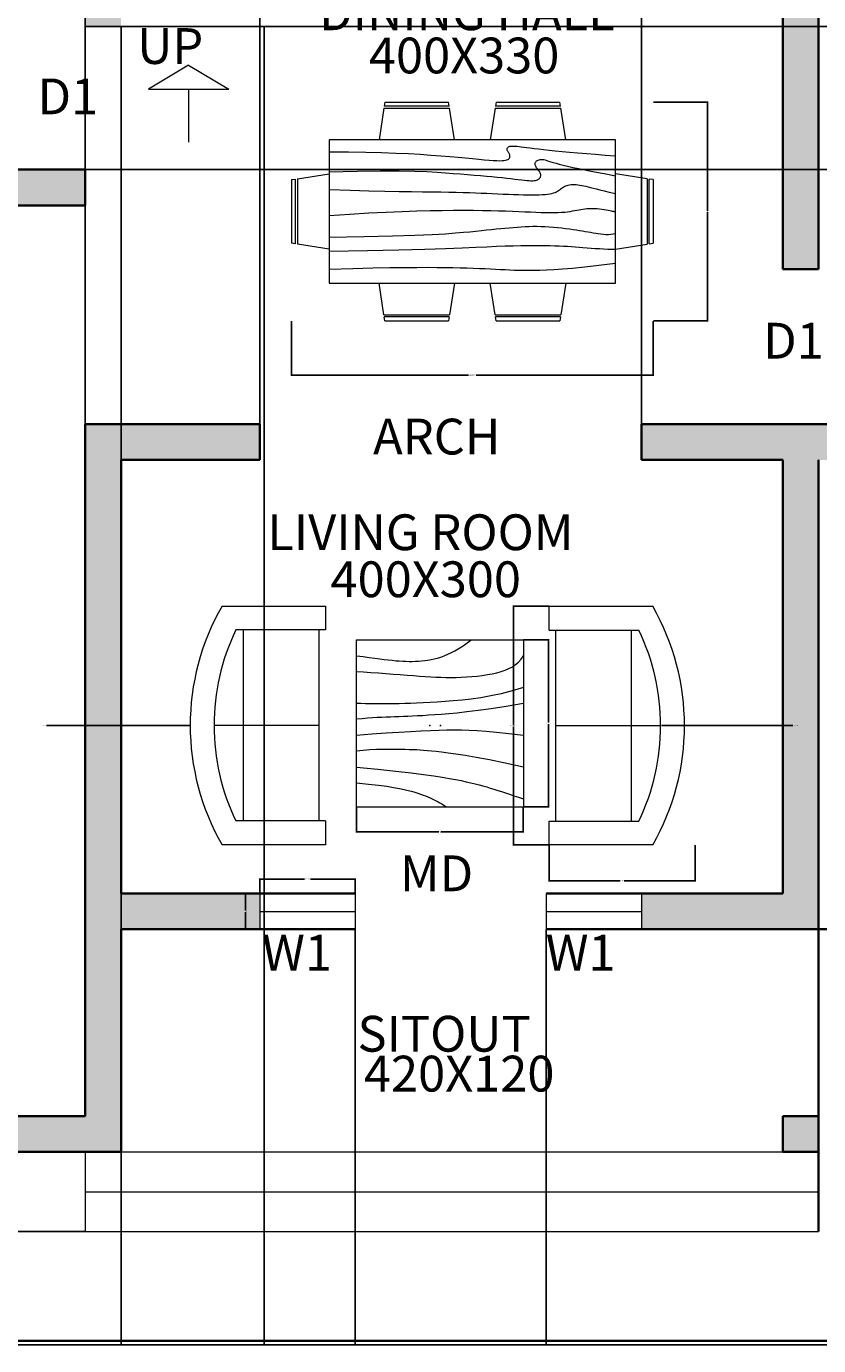
# Model space of a CAD drawing. Units: inches. Extents: x 1332 to 3175, y 1481 to 2088.
# Tile 2 of 5: x 1518 to 1717, y 1484 to 1816. Entities that reach past the tile are written whole.
import ezdxf

# ---------------------------------------------------------------- set-up
doc = ezdxf.new("R2010")
doc.units = ezdxf.units.IN
for name, color, linetype, lineweight in [('A-ANNO-DIMS', 2, 'Continuous', 18), ('A-ANNO-SYMB', 7, 'Continuous', 18), ('A-ANNO-TEXT', 7, 'Continuous', 18), ('A-ANNO-TTLB', 7, 'Continuous', 35), ('A-AREA-IDEN', 7, 'Continuous', 18), ('A-FLOR-STRS', 7, 'Continuous', 18), ('A-FURN', 8, 'Continuous', 18), ('A-WALL', 7, 'Continuous', 35)]:
    doc.layers.add(name, color=color, linetype=linetype, lineweight=lineweight)
for name, color, linetype, lineweight, true_color in [('A-COLS', 18, 'Continuous', 35, 0x000000), ('A-GLAZ', 30, 'Continuous', 18, 0xf8991e), ('A-WALL-PATT', 18, 'Continuous', 13, 0x000000)]:
    doc.layers.add(name, color=color, linetype=linetype, lineweight=lineweight, true_color=true_color)
doc.styles.get("Standard").update_dxf_attribs({"font": 'arial.ttf'})
doc.dimstyles.get("Standard").update_dxf_attribs({"dimtxt": 0.18, "dimasz": 0.18, "dimexe": 0.18, "dimexo": 0.0625, "dimgap": 0.09, "dimtad": 0, "dimtih": 1, "dimtoh": 1, "dimdec": 4, "dimzin": 0, "dimdsep": 46, "dimtxsty": 'Standard', "dimcen": 0.09, "dimadec": 0, "dimazin": 0, "dimtfac": 1, "dimtdec": 4, "dimtofl": 0, "dimtmove": 0, "dimatfit": 3, "dimfxl": 1, "dimtolj": 1, "dimtzin": 0, "dimarcsym": 0})

# ---------------------------------------------------------------- blocks, each defined once
blk = doc.blocks.new('Sofa - Roundback Loveseat 5 ft.')
for p, q in [((0, -32.44198), (0, -5.99998)), ((-24, -33.99998), (-24, -11.46958)), ((24.00004, -33.99998), (24.00004, -11.46958)), ((-23.9998, -13.38178), (23.99986, -13.38178)), ((-24, -32.44198), (24.00004, -32.44198))]:
    blk.add_line(p, q)
for points in [[(-24, -33.99998), (-30, -33.99998), (-30, -7.99998)], [(30.00004, -7.99998), (30.00004, -33.99998), (24.00004, -33.99998)]]:
    blk.add_lwpolyline(points)
for centre, radius, start, end in [((0, -60.24998), 60.24998, 60.13715, 119.8628), ((0, -61.38438), 55.38444, 64.32083, 115.6792)]:
    blk.add_arc(centre, radius, start, end)
blk = doc.blocks.new('Table - Square Woodgrain 42 x 42 in.')
blk.add_line((0, -42), (42, -42))
for points in [[(0, -4), (1.704, -4.2172), (3.2358, -4.4188), (4.615, -4.604), (5.8615, -4.7721), (6.9951, -4.9224), (8.0357, -5.0541), (9.0031, -5.1667), (9.9171, -5.2594), (10.7951, -5.3316), (11.6445, -5.3836), (12.4702, -5.4157), (13.277, -5.4283), (14.0698, -5.4217), (14.8535, -5.3964), (15.6331, -5.3526), (16.4133, -5.2908), (17.1986, -5.2103), (17.9913, -5.1062), (18.793, -4.9727), (19.6056, -4.8038), (20.4307, -4.5937), (21.2701, -4.3365), (22.1256, -4.0262), (22.9989, -3.6571), (23.888, -3.2272), (24.7756, -2.7516), (25.6408, -2.2491), (26.4624, -1.7387), (27.2195, -1.2395), (27.891, -0.7703), (28.456, -0.3501), (28.8934, 0.002)], [(0, -42), (0, 0), (42, 0), (42, -42)], [(0, -8), (1.8203, -8.1001), (3.6741, -8.2149), (5.5411, -8.3408), (7.4011, -8.4741), (9.2339, -8.6112), (11.0193, -8.7484), (12.7371, -8.8821), (14.3671, -9.0086), (15.8954, -9.1246), (17.3337, -9.2278), (18.6997, -9.3159), (20.0116, -9.387), (21.2871, -9.4389), (22.5442, -9.4696), (23.8008, -9.477), (25.0749, -9.459), (26.3791, -9.4137), (27.7049, -9.3403), (29.0383, -9.2382), (30.3655, -9.1068), (31.6728, -8.9455), (32.9461, -8.7535), (34.1717, -8.5304), (35.3358, -8.2756), (36.4268, -7.9863), (37.443, -7.6521), (38.3849, -7.2603), (39.253, -6.7986), (40.048, -6.2542), (40.7705, -5.6147), (41.421, -4.8674), (42, -4)], [(42, -12), (39.1784, -12.8621), (36.4519, -13.5654), (33.8246, -14.1294), (31.3004, -14.5731), (28.8832, -14.9161), (26.577, -15.1775), (24.3858, -15.3768), (22.3136, -15.5332), (20.3622, -15.6632), (18.5254, -15.7718), (16.7947, -15.8612), (15.1618, -15.9338), (13.6183, -15.9916), (12.1558, -16.0369), (10.7659, -16.0718), (9.4403, -16.0987), (8.1703, -16.1191), (6.9461, -16.1325), (5.7577, -16.1377), (4.595, -16.1335), (3.4479, -16.1188), (2.3064, -16.0924), (1.1604, -16.0532), (0, -16)], [(42, -16), (37.6529, -16.7365), (33.8802, -17.329), (30.6179, -17.7961), (27.8015, -18.1561), (25.3668, -18.4275), (23.2497, -18.6288), (21.3859, -18.7785), (19.7111, -18.8949), (18.1693, -18.9939), (16.7375, -19.0795), (15.401, -19.1534), (14.1449, -19.217), (12.9544, -19.2717), (11.8148, -19.3191), (10.7113, -19.3606), (9.6291, -19.3976), (8.5534, -19.4323), (7.47, -19.4689), (6.3643, -19.5122), (5.222, -19.5672), (4.0288, -19.6386), (2.7703, -19.7313), (1.4321, -19.8501), (0, -20)], [(0, -24), (3.9243, -23.6805), (7.4766, -23.4138), (10.6891, -23.1954), (13.5943, -23.0205), (16.2247, -22.8847), (18.6125, -22.7832), (20.7903, -22.7116), (22.7903, -22.6651), (24.6563, -22.642), (26.4764, -22.6507), (28.35, -22.7024), (30.3766, -22.8084), (32.6555, -22.98), (35.2861, -23.2283), (38.3678, -23.5645), (42, -24)], [(42, -32), (37.392, -31.017), (33.4585, -30.2231), (30.1291, -29.5949), (27.3334, -29.109), (25.0009, -28.742), (23.0612, -28.4707), (21.4439, -28.2716), (20.0786, -28.1215), (18.8998, -28.0002), (17.8609, -27.9014), (16.9206, -27.8219), (16.0371, -27.7588), (15.1691, -27.709), (14.2748, -27.6693), (13.3128, -27.6368), (12.2415, -27.6083), (11.0295, -27.5824), (9.6867, -27.5643), (8.233, -27.5608), (6.6884, -27.5787), (5.0728, -27.6248), (3.4062, -27.7058), (1.7086, -27.8286), (0, -28)], [(0, -32), (5.4026, -32.5358), (9.9494, -33.019), (13.7424, -33.4553), (16.8834, -33.8505), (19.4743, -34.2106), (21.6171, -34.5413), (23.4136, -34.8486), (24.9657, -35.1382), (26.3614, -35.4156), (27.6332, -35.6841), (28.7995, -35.9467), (29.8788, -36.2064), (30.8897, -36.4661), (31.8507, -36.7288), (32.7802, -36.9973), (33.6968, -37.2747), (34.6175, -37.5635), (35.5531, -37.8651), (36.5128, -38.1805), (37.506, -38.5108), (38.5421, -38.8568), (39.6302, -39.2197), (40.7797, -39.6004), (42, -40)], [(0, -36), (3.0098, -36.2857), (5.5354, -36.5643), (7.6368, -36.8359), (9.374, -37.1009), (10.807, -37.3597), (11.9957, -37.6126), (13.0002, -37.8599), (13.8804, -38.102), (14.6874, -38.3393), (15.4365, -38.5729), (16.1338, -38.8041), (16.7858, -39.0341), (17.3987, -39.264), (17.9787, -39.4952), (18.5322, -39.7288), (19.0655, -39.9662), (19.5832, -40.2081), (20.0842, -40.4544), (20.5657, -40.7046), (21.0249, -40.9581), (21.459, -41.2144), (21.8653, -41.4731), (22.2409, -41.7335), (22.5831, -41.9951)]]:
    blk.add_lwpolyline(points)
blk = doc.blocks.new('Dining Set - 36 x 72 in.')
for p, q in [((-22, 27.5), (-22.1562, 26.50042)), ((-22, 27.5), (-6, 27.5)), ((-5.8437, 26.49966), (-6, 27.5)), ((6, 27.5), (5.8438, 26.50042)), ((6, 27.5), (22, 27.5)), ((22.1563, 26.49966), (22, 27.5)), ((-22.2343, 26.00059), (-23.4847, 17.99762)), ((-22.2304, 26), (-5.7608, 26)), ((-5.8416, 26.5), (-22.1534, 26.5)), ((-4.5152, 17.99762), (-5.7655, 25.99926)), ((5.7657, 26.00059), (4.5153, 17.99762)), ((5.7696, 26), (22.2392, 26)), ((22.1584, 26.5), (5.8466, 26.5)), ((23.4848, 17.99762), (22.2345, 25.99926)), ((36, 18), (-36, 18)), ((-36, 18), (-36, -18)), ((36, -18), (36, 18)), ((-45.5, 8), (-44.5004, 8.15617)), ((-45.5, 8), (-45.5, -8)), ((-44.5, -8.15843), (-44.5, 8.15338)), ((-44.0006, 8.23428), (-35.9976, 9.48474)), ((-44, 8.23041), (-44, -8.23915)), ((44.0006, 8.23428), (35.9976, 9.48474)), ((44, 8.23041), (44, -8.23915)), ((44.5, -8.15843), (44.5, 8.15338)), ((45.5, 8), (44.5005, 8.15617)), ((45.5, 8), (45.5, -8)), ((-44.4997, -8.15631), (-45.5, -8)), ((-35.9976, -9.48476), (-43.9993, -8.2345)), ((35.9976, -9.48476), (43.9993, -8.2345)), ((44.4997, -8.15631), (45.5, -8)), ((-36, -18), (36, -18)), ((-22.2343, -26.0006), (-23.4847, -17.99762)), ((-4.5152, -17.99762), (-5.7655, -25.99928)), ((5.7657, -26.0006), (4.5153, -17.99762)), ((23.4848, -17.99762), (22.2345, -25.99928)), ((-22.2304, -26), (-5.7608, -26)), ((-22, -27.5), (-22.1562, -26.50044)), ((-5.8416, -26.5), (-22.1534, -26.5)), ((-5.8437, -26.49967), (-6, -27.5)), ((5.7696, -26), (22.2392, -26)), ((6, -27.5), (5.8438, -26.50044)), ((22.1584, -26.5), (5.8466, -26.5)), ((22.1563, -26.49967), (22, -27.5)), ((-22, -27.5), (-6, -27.5)), ((6, -27.5), (22, -27.5))]:
    blk.add_line(p, q)
for points in [[(-36, 15), (-31.1772, 14.97754), (-26.8079, 14.91406), (-22.8538, 14.81543), (-19.276, 14.6875), (-16.0362, 14.53613), (-13.0957, 14.36718), (-10.4159, 14.18652), (-7.9583, 14), (-5.6904, 13.81315), (-3.6035, 13.63021), (-1.6954, 13.45508), (0.0365, 13.29166), (1.5945, 13.14388), (2.9811, 13.01562), (4.1988, 12.9108), (5.25, 12.83333), (6.1393, 12.78613), (6.8802, 12.76823), (7.4883, 12.77767), (7.9792, 12.8125), (8.3685, 12.87077), (8.6719, 12.95052), (8.9049, 13.0498), (9.0833, 13.16666), (9.2205, 13.29899), (9.3216, 13.44401), (9.3895, 13.59879), (9.4271, 13.76041), (9.4373, 13.92594), (9.4232, 14.09245), (9.3875, 14.257), (9.3333, 14.41666), (9.2638, 14.56917), (9.1836, 14.71484), (9.0975, 14.85465), (9.0104, 14.98958), (8.9272, 15.1206), (8.8529, 15.2487), (8.7922, 15.37483), (8.75, 15.5), (8.7305, 15.62467), (8.7344, 15.74739), (8.7617, 15.86621), (8.8125, 15.97916), (8.8867, 16.08431), (8.9844, 16.17968), (9.1055, 16.26334), (9.25, 16.33333), (9.4189, 16.38802), (9.6172, 16.42708), (9.8506, 16.45052), (10.125, 16.45833), (10.4463, 16.45052), (10.8203, 16.42708), (11.2529, 16.38802), (11.75, 16.33333), (12.3184, 16.26318), (12.9694, 16.17838), (13.7151, 16.07991), (14.5677, 15.96875), (15.5395, 15.84586), (16.6426, 15.71224), (17.8893, 15.56884), (19.2917, 15.41666), (20.859, 15.25667), (22.5879, 15.08984), (24.4721, 14.91715), (26.5052, 14.73958), (28.6809, 14.5581), (30.9929, 14.3737), (33.4347, 14.18733), (36, 14)], [(-36, 10), (-28.9766, 10.14274), (-23.1725, 10.20442), (-18.4241, 10.19775), (-14.5677, 10.13541), (-11.4399, 10.03011), (-8.877, 9.89453), (-6.7154, 9.74137), (-4.7917, 9.58333), (-2.9698, 9.43082), (-1.2246, 9.28515), (0.4415, 9.14534), (2.026, 9.01041), (3.5266, 8.87939), (4.9408, 8.7513), (6.266, 8.62516), (7.5, 8.5), (8.6411, 8.37549), (9.6914, 8.2539), (10.6538, 8.13818), (11.5312, 8.03125), (12.3267, 7.93603), (13.043, 7.85547), (13.6831, 7.79248), (14.25, 7.75), (14.7471, 7.7303), (15.1797, 7.73307), (15.5537, 7.75732), (15.875, 7.80208), (16.1494, 7.86637), (16.3828, 7.94922), (16.5811, 8.04964), (16.75, 8.16666), (16.8944, 8.29915), (17.0143, 8.44531), (17.1089, 8.60319), (17.1771, 8.77083), (17.218, 8.94629), (17.2305, 9.1276), (17.2137, 9.31282), (17.1667, 9.5), (17.0895, 9.6875), (16.987, 9.875), (16.8649, 10.0625), (16.7292, 10.25), (16.5856, 10.4375), (16.4401, 10.625), (16.2985, 10.8125), (16.1667, 11), (16.05, 11.18733), (15.9518, 11.3737), (15.8752, 11.5581), (15.8229, 11.73958), (15.798, 11.91715), (15.8034, 12.08984), (15.842, 12.25667), (15.9167, 12.41666), (16.0295, 12.56836), (16.1784, 12.70833), (16.3605, 12.83268), (16.5729, 12.9375), (16.8127, 13.01888), (17.0768, 13.07291), (17.3625, 13.0957), (17.6667, 13.08333), (17.9894, 13.03312), (18.3418, 12.94726), (18.7382, 12.82918), (19.1927, 12.68229), (19.7195, 12.51001), (20.3327, 12.31575), (21.0465, 12.10294), (21.875, 11.875), (22.8357, 11.63354), (23.959, 11.37304), (25.2786, 11.08618), (26.8282, 10.76562), (28.6414, 10.40405), (30.752, 9.99414), (33.1936, 9.52856), (36, 9)], [(-36, 5.5), (-30.7157, 5.3348), (-26.069, 5.20963), (-21.9946, 5.11767), (-18.4271, 5.05208), (-15.3009, 5.00602), (-12.5508, 4.97265), (-10.1112, 4.94515), (-7.9167, 4.91666), (-5.909, 4.88167), (-4.0586, 4.83984), (-2.3429, 4.79215), (-0.7396, 4.73958), (0.7739, 4.6831), (2.22, 4.6237), (3.6213, 4.56233), (5, 4.5), (6.373, 4.43782), (7.7344, 4.3776), (9.0723, 4.32129), (10.375, 4.27083), (11.6309, 4.22819), (12.8281, 4.19531), (13.9551, 4.17415), (15, 4.16666), (15.954, 4.17448), (16.819, 4.19791), (17.6001, 4.23698), (18.3021, 4.29166), (18.9299, 4.36198), (19.4883, 4.44791), (19.9823, 4.54948), (20.4167, 4.66666), (20.7969, 4.79899), (21.1302, 4.94401), (21.4245, 5.09879), (21.6875, 5.26041), (21.9271, 5.42594), (22.1511, 5.59245), (22.3672, 5.757), (22.5834, 5.91666), (22.8065, 6.06868), (23.0404, 6.21093), (23.2879, 6.34147), (23.5521, 6.45833), (23.8358, 6.55957), (24.142, 6.64323), (24.4735, 6.70735), (24.8334, 6.75), (25.2235, 6.76969), (25.642, 6.76692), (26.0858, 6.74267), (26.5521, 6.69791), (27.0379, 6.63362), (27.5404, 6.55078), (28.0565, 6.45036), (28.5834, 6.33333), (29.1242, 6.19987), (29.7071, 6.04687), (30.3661, 5.87044), (31.1354, 5.66666), (32.0493, 5.43164), (33.142, 5.16146), (34.4475, 4.85221), (36, 4.5)], [(-36, -1), (-30.7915, -0.6591), (-26.0195, -0.38216), (-21.6519, -0.16284), (-17.6563, 0.00521), (-14.0005, 0.12833), (-10.6523, 0.21289), (-7.5796, 0.26522), (-4.75, 0.29166), (-2.134, 0.29793), (0.2878, 0.28711), (2.5317, 0.26163), (4.6146, 0.22396), (6.5529, 0.17651), (8.3633, 0.12174), (10.0623, 0.06209), (11.6667, 0), (13.1899, -0.06201), (14.6341, -0.1211), (15.9982, -0.17432), (17.2813, -0.21875), (18.4823, -0.25147), (19.6003, -0.26953), (20.6343, -0.27002), (21.5834, -0.25), (22.4481, -0.20768), (23.2357, -0.14584), (23.9549, -0.06836), (24.6146, 0.02083), (25.2235, 0.11784), (25.7904, 0.21875), (26.3241, 0.31966), (26.8334, 0.41666), (27.3265, 0.50618), (27.8099, 0.58593), (28.2894, 0.65397), (28.7709, 0.70833), (29.2601, 0.74707), (29.763, 0.76823), (30.2855, 0.76985), (30.8334, 0.75), (31.4088, 0.70784), (31.9994, 0.64713), (32.589, 0.57275), (33.1615, 0.48958), (33.7008, 0.4025), (34.1908, 0.3164), (34.6153, 0.23616), (34.9584, 0.16666), (35.2099, 0.11165), (35.3848, 0.07031), (35.504, 0.04069), (35.5886, 0.02083), (35.6594, 0.00879), (35.7377, 0.0026), (35.8442, 0.00032), (36, 0)], [(-36, -6.5), (-27.1843, -6.31267), (-20.084, -6.1263), (-14.469, -5.9419), (-10.1094, -5.76042), (-6.7752, -5.58285), (-4.2363, -5.41016), (-2.2629, -5.24333), (-0.625, -5.08334), (0.8708, -4.93099), (2.2715, -4.78646), (3.5872, -4.64974), (4.8281, -4.52084), (6.0046, -4.39974), (7.127, -4.28646), (8.2053, -4.18099), (9.25, -4.08334), (10.2705, -3.99382), (11.2734, -3.91407), (12.2647, -3.84603), (13.25, -3.79167), (14.2354, -3.75293), (15.2266, -3.73177), (16.2295, -3.73015), (17.25, -3.75), (18.2912, -3.79248), (19.3451, -3.85547), (20.4009, -3.93604), (21.4479, -4.03125), (22.4754, -4.13819), (23.4727, -4.25391), (24.4289, -4.37549), (25.3334, -4.5), (26.1785, -4.62492), (26.9694, -4.74935), (27.7145, -4.87281), (28.4219, -4.99479), (29.1, -5.11483), (29.7572, -5.23242), (30.4016, -5.34709), (31.0417, -5.45834), (31.6837, -5.56437), (32.3262, -5.65821), (32.9658, -5.73153), (33.599, -5.77604), (34.2224, -5.78345), (34.8327, -5.74545), (35.4264, -5.65373), (36, -5.5)], [(-36, -10), (-26.4022, -9.81299), (-18.4675, -9.62891), (-11.9839, -9.45069), (-6.7396, -9.28125), (-2.5226, -9.12354), (0.8789, -8.98047), (3.6769, -8.85498), (6.0833, -8.75), (8.2767, -8.66765), (10.3021, -8.60677), (12.1712, -8.56543), (13.8958, -8.54167), (15.4876, -8.53353), (16.9583, -8.53907), (18.3197, -8.55632), (19.5834, -8.58334), (20.7616, -8.61841), (21.8685, -8.66081), (22.9188, -8.71004), (23.9271, -8.76563), (24.9081, -8.82707), (25.8763, -8.89388), (26.8465, -8.96558), (27.8334, -9.04167), (28.8474, -9.12118), (29.8828, -9.20117), (30.93, -9.27824), (31.9792, -9.34896), (33.0205, -9.40991), (34.0443, -9.45768), (35.0407, -9.48885), (36, -9.5)], [(-36, -14.5), (-30.0881, -14.33513), (-25.0332, -14.21224), (-20.7312, -14.12647), (-17.0781, -14.07292), (-13.97, -14.04671), (-11.3027, -14.04297), (-8.9724, -14.05681), (-6.875, -14.08334), (-4.9224, -14.11833), (-3.0905, -14.16016), (-1.3709, -14.20785), (0.2448, -14.26042), (1.7647, -14.3169), (3.1973, -14.3763), (4.5507, -14.43767), (5.8333, -14.5), (7.0554, -14.5621), (8.235, -14.62175), (9.3922, -14.67652), (10.5469, -14.72396), (11.7192, -14.76164), (12.929, -14.78711), (14.1965, -14.79794), (15.5417, -14.79167), (16.9933, -14.76424), (18.6152, -14.70508), (20.4804, -14.60197), (22.6615, -14.44271), (25.2312, -14.21509), (28.2624, -13.9069), (31.8277, -13.50594), (36, -13)]]:
    blk.add_lwpolyline(points)
blk = doc.blocks.new('COL-SQUARE-9-PLAN')
h = blk.add_hatch(color=256)
h.dxf.hatch_style = 1
h.paths.add_polyline_path([(9, 9), (0, 9), (0, 0), (9, 0)])
blk.add_lwpolyline([(0, 9), (9, 9), (9, 0), (0, 0)], close=True)
blk = doc.blocks.new('WIN-W1-24')
for p, q in [((0, 9), (0, 0)), ((24, 9), (24, 0)), ((0, 4.5), (24, 4.5))]:
    blk.add_line(p, q)
blk = doc.blocks.new('*D21')
at = {"layer": 'A-ANNO-DIMS', "color": 0, "lineweight": -2, "transparency": 16777216}
for p, q in [((1649.32, 1670.31), (1640.2, 1670.31)), ((1640.38, 1670.13), (1640.38, 1640.49)), ((1640.38, 1610.49), (1640.38, 1640.13)), ((1649.32, 1610.31), (1640.2, 1610.31))]:
    blk.add_line(p, q, dxfattribs=at)
at = {"layer": 'A-ANNO-DIMS', "color": 0, "transparency": 16777216}
for points in [[(1640.35, 1670.13), (1640.41, 1670.13), (1640.38, 1670.31)], [(1640.35, 1610.49), (1640.41, 1610.49), (1640.38, 1610.31)]]:
    blk.add_solid(points, dxfattribs=at)
at = {"layer": 'Defpoints', "color": 0, "transparency": 16777216}
for p in [(1649.38, 1670.31), (1640.38, 1610.31), (1649.38, 1610.31)]:
    blk.add_point(p, dxfattribs=at)
at = {"layer": 'A-ANNO-DIMS', "color": 0, "transparency": 16777216, "insert": (1640.38, 1640.31), "char_height": 0.18, "attachment_point": 5}
blk.add_mtext('\\A1;LOVESEAT 60 TYP.', dxfattribs=at)
blk = doc.blocks.new('*D22')
at = {"layer": 'A-ANNO-DIMS', "color": 0, "lineweight": -2, "transparency": 16777216}
for p, q in [((1649.38, 1610.25), (1649.38, 1601.13)), ((1686.05, 1610.25), (1686.05, 1601.13)), ((1649.56, 1601.31), (1667.19, 1601.31)), ((1685.87, 1601.31), (1668.24, 1601.31))]:
    blk.add_line(p, q, dxfattribs=at)
at = {"layer": 'A-ANNO-DIMS', "color": 0, "transparency": 16777216}
for points in [[(1649.56, 1601.34), (1649.56, 1601.28), (1649.38, 1601.31)], [(1685.87, 1601.34), (1685.87, 1601.28), (1686.05, 1601.31)]]:
    blk.add_solid(points, dxfattribs=at)
at = {"layer": 'Defpoints', "color": 0, "transparency": 16777216}
for p in [(1649.38, 1610.31), (1686.05, 1610.31), (1686.05, 1601.31)]:
    blk.add_point(p, dxfattribs=at)
at = {"layer": 'A-ANNO-DIMS', "color": 0, "transparency": 16777216, "insert": (1667.71, 1601.31), "char_height": 0.18, "attachment_point": 5}
blk.add_mtext('\\A1;37 TYP.', dxfattribs=at)
blk = doc.blocks.new('*D25')
at = {"layer": 'A-ANNO-DIMS', "color": 0, "lineweight": -2, "transparency": 16777216}
for p, q in [((1576.56, 1598.18), (1576.56, 1601.9)), ((1576.74, 1601.72), (1587.81, 1601.72)), ((1600.38, 1601.72), (1589.32, 1601.72)), ((1600.56, 1598.18), (1600.56, 1601.9))]:
    blk.add_line(p, q, dxfattribs=at)
at = {"layer": 'A-ANNO-DIMS', "color": 0, "transparency": 16777216}
for points in [[(1576.74, 1601.75), (1576.74, 1601.69), (1576.56, 1601.72)], [(1600.38, 1601.75), (1600.38, 1601.69), (1600.56, 1601.72)]]:
    blk.add_solid(points, dxfattribs=at)
at = {"layer": 'Defpoints', "color": 0, "transparency": 16777216}
for p in [(1600.56, 1601.72), (1576.56, 1598.12), (1600.56, 1598.12)]:
    blk.add_point(p, dxfattribs=at)
at = {"layer": 'A-ANNO-DIMS', "color": 0, "transparency": 16777216, "insert": (1588.56, 1601.72), "char_height": 0.18, "attachment_point": 5}
blk.add_mtext('\\A1;W1 24 TYP.', dxfattribs=at)
blk = doc.blocks.new('*D26')
at = {"layer": 'A-ANNO-DIMS', "color": 0, "lineweight": -2, "transparency": 16777216}
for p, q in [((1576.5, 1598.12), (1572.78, 1598.12)), ((1572.96, 1597.94), (1572.96, 1593.8)), ((1572.96, 1589.3), (1572.96, 1593.44)), ((1576.5, 1589.12), (1572.78, 1589.12))]:
    blk.add_line(p, q, dxfattribs=at)
at = {"layer": 'A-ANNO-DIMS', "color": 0, "transparency": 16777216}
for points in [[(1572.93, 1597.94), (1572.99, 1597.94), (1572.96, 1598.12)], [(1572.93, 1589.3), (1572.99, 1589.3), (1572.96, 1589.12)]]:
    blk.add_solid(points, dxfattribs=at)
at = {"layer": 'Defpoints', "color": 0, "transparency": 16777216}
for p in [(1572.96, 1598.12), (1576.56, 1598.12), (1576.56, 1589.12)]:
    blk.add_point(p, dxfattribs=at)
at = {"layer": 'A-ANNO-DIMS', "color": 0, "transparency": 16777216, "insert": (1572.96, 1593.62), "char_height": 0.18, "attachment_point": 5}
blk.add_mtext('\\A1;9 TYP.', dxfattribs=at)
blk = doc.blocks.new('*D31')
at = {"layer": 'A-ANNO-DIMS', "color": 0, "lineweight": -2, "transparency": 16777216}
for p, q in [((1642.91, 1661.9), (1649.32, 1661.9)), ((1649.14, 1661.72), (1649.14, 1641.08)), ((1649.14, 1620.08), (1649.14, 1640.72)), ((1642.91, 1619.9), (1649.32, 1619.9))]:
    blk.add_line(p, q, dxfattribs=at)
at = {"layer": 'A-ANNO-DIMS', "color": 0, "transparency": 16777216}
for points in [[(1649.11, 1661.72), (1649.17, 1661.72), (1649.14, 1661.9)], [(1649.11, 1620.08), (1649.17, 1620.08), (1649.14, 1619.9)]]:
    blk.add_solid(points, dxfattribs=at)
at = {"layer": 'Defpoints', "color": 0, "transparency": 16777216}
for p in [(1642.84, 1661.9), (1649.14, 1661.9), (1642.84, 1619.9)]:
    blk.add_point(p, dxfattribs=at)
at = {"layer": 'A-ANNO-DIMS', "color": 0, "transparency": 16777216, "insert": (1649.14, 1640.9), "char_height": 0.18, "attachment_point": 5}
blk.add_mtext('\\A1;TABLE 42', dxfattribs=at)
blk = doc.blocks.new('*D32')
at = {"layer": 'A-ANNO-DIMS', "color": 0, "lineweight": -2, "transparency": 16777216}
for p, q in [((1600.84, 1619.84), (1600.84, 1613.42)), ((1642.84, 1619.84), (1642.84, 1613.42)), ((1601.02, 1613.6), (1621.62, 1613.6)), ((1642.66, 1613.6), (1622.06, 1613.6))]:
    blk.add_line(p, q, dxfattribs=at)
at = {"layer": 'A-ANNO-DIMS', "color": 0, "transparency": 16777216}
for points in [[(1601.02, 1613.63), (1601.02, 1613.57), (1600.84, 1613.6)], [(1642.66, 1613.63), (1642.66, 1613.57), (1642.84, 1613.6)]]:
    blk.add_solid(points, dxfattribs=at)
at = {"layer": 'Defpoints', "color": 0, "transparency": 16777216}
for p in [(1600.84, 1619.9), (1642.84, 1619.9), (1642.84, 1613.6)]:
    blk.add_point(p, dxfattribs=at)
at = {"layer": 'A-ANNO-DIMS', "color": 0, "transparency": 16777216, "insert": (1621.84, 1613.6), "char_height": 0.18, "attachment_point": 5}
blk.add_mtext('\\A1;42', dxfattribs=at)
blk = doc.blocks.new('*D33')
at = {"layer": 'A-ANNO-DIMS', "color": 0, "lineweight": -2, "transparency": 16777216}
for p, q in [((1584.52, 1742.02), (1584.52, 1728.25)), ((1675.52, 1742.02), (1675.52, 1728.25)), ((1584.7, 1728.43), (1629.07, 1728.43)), ((1675.34, 1728.43), (1630.97, 1728.43))]:
    blk.add_line(p, q, dxfattribs=at)
at = {"layer": 'A-ANNO-DIMS', "color": 0, "transparency": 16777216}
for points in [[(1584.7, 1728.46), (1584.7, 1728.4), (1584.52, 1728.43)], [(1675.34, 1728.46), (1675.34, 1728.4), (1675.52, 1728.43)]]:
    blk.add_solid(points, dxfattribs=at)
at = {"layer": 'Defpoints', "color": 0, "transparency": 16777216}
for p in [(1584.52, 1742.08), (1675.52, 1742.08), (1675.52, 1728.43)]:
    blk.add_point(p, dxfattribs=at)
at = {"layer": 'A-ANNO-DIMS', "color": 0, "transparency": 16777216, "insert": (1630.02, 1728.43), "char_height": 0.18, "attachment_point": 5}
blk.add_mtext('\\A1;DINING SET 91', dxfattribs=at)
blk = doc.blocks.new('*D34')
at = {"layer": 'A-ANNO-DIMS', "color": 0, "lineweight": -2, "transparency": 16777216}
for p, q in [((1675.58, 1797.08), (1689.35, 1797.08)), ((1689.17, 1796.9), (1689.17, 1769.77)), ((1689.17, 1742.26), (1689.17, 1769.4)), ((1675.58, 1742.08), (1689.35, 1742.08))]:
    blk.add_line(p, q, dxfattribs=at)
at = {"layer": 'A-ANNO-DIMS', "color": 0, "transparency": 16777216}
for points in [[(1689.14, 1796.9), (1689.2, 1796.9), (1689.17, 1797.08)], [(1689.14, 1742.26), (1689.2, 1742.26), (1689.17, 1742.08)]]:
    blk.add_solid(points, dxfattribs=at)
at = {"layer": 'Defpoints', "color": 0, "transparency": 16777216}
for p in [(1675.52, 1797.08), (1689.17, 1797.08), (1675.52, 1742.08)]:
    blk.add_point(p, dxfattribs=at)
at = {"layer": 'A-ANNO-DIMS', "color": 0, "transparency": 16777216, "insert": (1689.17, 1769.58), "char_height": 0.18, "attachment_point": 5}
blk.add_mtext('\\A1;55', dxfattribs=at)
blk = doc.blocks.new('*D37')
at = {"layer": 'A-ANNO-DIMS', "color": 0, "lineweight": -2, "transparency": 16777216}
for p, q in [((1851.13, 1589.06), (1851.13, 1484.44)), ((1389.63, 1533.06), (1389.63, 1484.44)), ((1389.81, 1484.62), (1619.98, 1484.62)), ((1850.95, 1484.62), (1620.78, 1484.62))]:
    blk.add_line(p, q, dxfattribs=at)
at = {"layer": 'A-ANNO-DIMS', "color": 0, "transparency": 16777216}
for points in [[(1389.81, 1484.65), (1389.81, 1484.59), (1389.63, 1484.62)], [(1850.95, 1484.65), (1850.95, 1484.59), (1851.13, 1484.62)]]:
    blk.add_solid(points, dxfattribs=at)
at = {"layer": 'Defpoints', "color": 0, "transparency": 16777216}
for p in [(1851.13, 1589.12), (1389.63, 1533.12), (1851.13, 1484.62)]:
    blk.add_point(p, dxfattribs=at)
at = {"layer": 'A-ANNO-DIMS', "color": 0, "transparency": 16777216, "insert": (1620.38, 1484.62), "char_height": 0.18, "attachment_point": 5}
blk.add_mtext('\\A1;461.5', dxfattribs=at)
blk = doc.blocks.new('*D38')
at = {"layer": 'A-ANNO-DIMS', "color": 0, "lineweight": -2, "transparency": 16777216}
for p, q in [((1444.57, 1991.12), (1360.95, 1991.12)), ((1361.13, 1990.94), (1361.13, 1752.3)), ((1361.13, 1513.3), (1361.13, 1751.94)), ((1532.57, 1513.12), (1360.95, 1513.12))]:
    blk.add_line(p, q, dxfattribs=at)
at = {"layer": 'A-ANNO-DIMS', "color": 0, "transparency": 16777216}
for points in [[(1361.1, 1990.94), (1361.16, 1990.94), (1361.13, 1991.12)], [(1361.1, 1513.3), (1361.16, 1513.3), (1361.13, 1513.12)]]:
    blk.add_solid(points, dxfattribs=at)
at = {"layer": 'Defpoints', "color": 0, "transparency": 16777216}
for p in [(1361.13, 1991.12), (1444.63, 1991.12), (1532.63, 1513.12)]:
    blk.add_point(p, dxfattribs=at)
at = {"layer": 'A-ANNO-DIMS', "color": 0, "transparency": 16777216, "insert": (1361.13, 1752.12), "char_height": 0.18, "attachment_point": 5}
blk.add_mtext('\\A1;478', dxfattribs=at)
blk = doc.blocks.new('*D83')
at = {"layer": 'A-ANNO-DIMS', "color": 0, "lineweight": -2, "transparency": 16777216}
for p, q in [((1600.56, 1589.06), (1600.56, 1484.44)), ((1648.56, 1589.06), (1648.56, 1484.44)), ((1600.74, 1484.62), (1624.34, 1484.62)), ((1648.38, 1484.62), (1624.78, 1484.62))]:
    blk.add_line(p, q, dxfattribs=at)
at = {"layer": 'A-ANNO-DIMS', "color": 0, "transparency": 16777216}
for points in [[(1600.74, 1484.65), (1600.74, 1484.59), (1600.56, 1484.62)], [(1648.38, 1484.65), (1648.38, 1484.59), (1648.56, 1484.62)]]:
    blk.add_solid(points, dxfattribs=at)
at = {"layer": 'Defpoints', "color": 0, "transparency": 16777216}
for p in [(1600.56, 1589.12), (1648.56, 1589.12), (1648.56, 1484.62)]:
    blk.add_point(p, dxfattribs=at)
at = {"layer": 'A-ANNO-DIMS', "color": 0, "transparency": 16777216, "insert": (1624.56, 1484.62), "char_height": 0.18, "attachment_point": 5}
blk.add_mtext('\\A1;48', dxfattribs=at)
blk = doc.blocks.new('*D84')
at = {"layer": 'A-ANNO-DIMS', "color": 0, "lineweight": -2, "transparency": 16777216}
for p, q in [((1576.56, 1716.18), (1576.56, 2019.8)), ((1576.74, 2019.62), (1624.34, 2019.62)), ((1672.38, 2019.62), (1624.78, 2019.62)), ((1672.56, 1716.18), (1672.56, 2019.8))]:
    blk.add_line(p, q, dxfattribs=at)
at = {"layer": 'A-ANNO-DIMS', "color": 0, "transparency": 16777216}
for points in [[(1576.74, 2019.65), (1576.74, 2019.59), (1576.56, 2019.62)], [(1672.38, 2019.65), (1672.38, 2019.59), (1672.56, 2019.62)]]:
    blk.add_solid(points, dxfattribs=at)
at = {"layer": 'Defpoints', "color": 0, "transparency": 16777216}
for p in [(1672.56, 2019.62), (1576.56, 1716.12), (1672.56, 1716.12)]:
    blk.add_point(p, dxfattribs=at)
at = {"layer": 'A-ANNO-DIMS', "color": 0, "transparency": 16777216, "insert": (1624.56, 2019.62), "char_height": 0.18, "attachment_point": 5}
blk.add_mtext('\\A1;96', dxfattribs=at)
blk = doc.blocks.new('*D87')
at = {"layer": 'A-ANNO-DIMS', "color": 0, "lineweight": -2, "transparency": 16777216}
for p, q in [((1493.63, 1716.18), (1493.63, 2019.8)), ((1493.81, 2019.62), (1512.91, 2019.62)), ((1532.45, 2019.62), (1513.35, 2019.62)), ((1532.63, 1716.18), (1532.63, 2019.8))]:
    blk.add_line(p, q, dxfattribs=at)
at = {"layer": 'A-ANNO-DIMS', "color": 0, "transparency": 16777216}
for points in [[(1493.81, 2019.65), (1493.81, 2019.59), (1493.63, 2019.62)], [(1532.45, 2019.65), (1532.45, 2019.59), (1532.63, 2019.62)]]:
    blk.add_solid(points, dxfattribs=at)
at = {"layer": 'Defpoints', "color": 0, "transparency": 16777216}
for p in [(1532.63, 2019.62), (1493.63, 1716.12), (1532.63, 1716.12)]:
    blk.add_point(p, dxfattribs=at)
at = {"layer": 'A-ANNO-DIMS', "color": 0, "transparency": 16777216, "insert": (1513.13, 2019.62), "char_height": 0.18, "attachment_point": 5}
blk.add_mtext('\\A1;39', dxfattribs=at)
blk = doc.blocks.new('*D88')
at = {"layer": 'A-ANNO-DIMS', "color": 0, "lineweight": -2, "transparency": 16777216}
for p, q in [((1532.69, 1816.12), (1879.81, 1816.12)), ((1879.63, 1815.94), (1879.63, 1798.3)), ((1879.63, 1780.3), (1879.63, 1797.94)), ((1532.69, 1780.12), (1879.81, 1780.12))]:
    blk.add_line(p, q, dxfattribs=at)
at = {"layer": 'A-ANNO-DIMS', "color": 0, "transparency": 16777216}
for points in [[(1879.6, 1815.94), (1879.66, 1815.94), (1879.63, 1816.12)], [(1879.6, 1780.3), (1879.66, 1780.3), (1879.63, 1780.12)]]:
    blk.add_solid(points, dxfattribs=at)
at = {"layer": 'Defpoints', "color": 0, "transparency": 16777216}
for p in [(1532.63, 1816.12), (1879.63, 1816.12), (1532.63, 1780.12)]:
    blk.add_point(p, dxfattribs=at)
at = {"layer": 'A-ANNO-DIMS', "color": 0, "transparency": 16777216, "insert": (1879.63, 1798.12), "char_height": 0.18, "attachment_point": 5}
blk.add_mtext('\\A1;36', dxfattribs=at)
blk = doc.blocks.new('*D89')
at = {"layer": 'A-ANNO-DIMS', "color": 0, "lineweight": -2, "transparency": 16777216}
for p, q in [((1541.63, 1816.06), (1541.63, 1484.44)), ((1577.63, 1816.06), (1577.63, 1484.44)), ((1541.81, 1484.62), (1559.41, 1484.62)), ((1577.45, 1484.62), (1559.85, 1484.62))]:
    blk.add_line(p, q, dxfattribs=at)
at = {"layer": 'A-ANNO-DIMS', "color": 0, "transparency": 16777216}
for points in [[(1541.81, 1484.65), (1541.81, 1484.59), (1541.63, 1484.62)], [(1577.45, 1484.65), (1577.45, 1484.59), (1577.63, 1484.62)]]:
    blk.add_solid(points, dxfattribs=at)
at = {"layer": 'Defpoints', "color": 0, "transparency": 16777216}
for p in [(1541.63, 1816.12), (1577.63, 1816.12), (1577.63, 1484.62)]:
    blk.add_point(p, dxfattribs=at)
at = {"layer": 'A-ANNO-DIMS', "color": 0, "transparency": 16777216, "insert": (1559.63, 1484.62), "char_height": 0.18, "attachment_point": 5}
blk.add_mtext('\\A1;36', dxfattribs=at)
blk = doc.blocks.new('*D90')
at = {"layer": 'A-ANNO-DIMS', "color": 0, "lineweight": -2, "transparency": 16777216}
for p, q in [((1522.89, 1640.36), (1558.86, 1640.36)), ((1619.2, 1640.36), (1619.38, 1640.36)), ((1619.29, 1640.27), (1619.29, 1640.45))]:
    blk.add_line(p, q, dxfattribs=at)
at = {"layer": 'A-ANNO-DIMS', "color": 0, "transparency": 16777216}
blk.add_solid([(1558.86, 1640.39), (1558.86, 1640.33), (1559.04, 1640.36)], dxfattribs=at)
at = {"layer": 'Defpoints', "color": 0, "transparency": 16777216}
for p in [(1559.04, 1640.36), (1619.29, 1640.36)]:
    blk.add_point(p, dxfattribs=at)
at = {"layer": 'A-ANNO-DIMS', "color": 0, "transparency": 16777216, "insert": (1522.21, 1640.36), "char_height": 0.18, "attachment_point": 5}
blk.add_mtext('\\A1;2X R60.25', dxfattribs=at)
blk = doc.blocks.new('*D91')
at = {"layer": 'A-ANNO-DIMS', "color": 0, "lineweight": -2, "transparency": 16777216}
for p, q in [((1621.91, 1640.31), (1622.09, 1640.31)), ((1622, 1640.22), (1622, 1640.4)), ((1710.61, 1640.31), (1677.56, 1640.31))]:
    blk.add_line(p, q, dxfattribs=at)
at = {"layer": 'A-ANNO-DIMS', "color": 0, "transparency": 16777216}
blk.add_solid([(1677.56, 1640.34), (1677.56, 1640.28), (1677.38, 1640.31)], dxfattribs=at)
at = {"layer": 'Defpoints', "color": 0, "transparency": 16777216}
for p in [(1622, 1640.31), (1677.38, 1640.31)]:
    blk.add_point(p, dxfattribs=at)
at = {"layer": 'A-ANNO-DIMS', "color": 0, "transparency": 16777216, "insert": (1711.29, 1640.31), "char_height": 0.18, "attachment_point": 5}
blk.add_mtext('\\A1;2X R55.38', dxfattribs=at)

msp = doc.modelspace()

# ---------------------------------------------------------------- hatches: boundary and pattern name
at = {"layer": 'A-WALL-PATT'}
h = msp.add_hatch(color=256, dxfattribs=at)
h.dxf.hatch_style = 1
h.paths.add_polyline_path([(1398.6316, 1914.1183), (1442.6316, 1914.1183), (1442.6316, 1923.1183), (1389.6316, 1923.1183), (1389.6316, 1868.1183), (1398.6316, 1868.1183)])
h.paths.add_polyline_path([(1398.6316, 1828.1183), (1389.6316, 1828.1183), (1389.6316, 1759.1183), (1398.6316, 1759.1183), (1398.6316, 1771.1183), (1477.6316, 1771.1183), (1477.6316, 1716.1183), (1437.6316, 1716.1183), (1437.6316, 1707.1183), (1493.6316, 1707.1183), (1493.6316, 1716.1183), (1486.6316, 1716.1183), (1486.6316, 1771.1183), (1532.6316, 1771.1183), (1532.6316, 1780.1183), (1398.6316, 1780.1183)])
h.paths.add_polyline_path([(1398.6316, 1735.1183), (1389.6316, 1735.1183), (1389.6316, 1647.6183), (1398.6316, 1647.6183)])
h.paths.add_polyline_path([(1398.6316, 1599.6183), (1389.6316, 1599.6183), (1389.6316, 1533.1183), (1442.6316, 1533.1183), (1442.6316, 1542.1183), (1398.6316, 1542.1183)])
h.paths.add_polyline_path([(1541.6316, 1589.1183), (1576.5616, 1589.1183), (1576.5616, 1598.1183), (1541.6316, 1598.1183), (1541.6316, 1707.1183), (1576.5616, 1707.1183), (1576.5616, 1716.1183), (1532.6316, 1716.1183), (1532.6316, 1542.1183), (1490.6316, 1542.1183), (1490.6316, 1533.1183), (1541.6316, 1533.1183)])
h.paths.add_polyline_path([(1717.1316, 1707.1183), (1752.1316, 1707.1183), (1752.1316, 1716.1183), (1672.5616, 1716.1183), (1672.5616, 1707.1183), (1708.1316, 1707.1183), (1708.1316, 1598.1183), (1672.5616, 1598.1183), (1672.5616, 1589.1183), (1717.1316, 1589.1183)])
h.paths.add_polyline_path([(1851.1316, 1761.1183), (1842.1316, 1761.1183), (1842.1316, 1716.1183), (1800.1316, 1716.1183), (1800.1316, 1707.1183), (1851.1316, 1707.1183)])
h.paths.add_polyline_path([(1851.1316, 1855.1183), (1784.1316, 1855.1183), (1784.1316, 1923.1183), (1750.1316, 1923.1183), (1750.1316, 1914.1183), (1775.1316, 1914.1183), (1775.1316, 1855.1183), (1750.1316, 1855.1183), (1750.1316, 1846.1183), (1842.1316, 1846.1183), (1842.1316, 1801.1183), (1851.1316, 1801.1183)])
h.paths.add_polyline_path([(1717.1316, 1914.1183), (1726.1316, 1914.1183), (1726.1316, 1923.1183), (1673.1316, 1923.1183), (1673.1316, 1914.1183), (1708.1316, 1914.1183), (1708.1316, 1755.1183), (1717.1316, 1755.1183)])
h.paths.add_polyline_path([(1661.1316, 1855.1183), (1636.1316, 1855.1183), (1636.1316, 1914.1183), (1649.1316, 1914.1183), (1649.1316, 1923.1183), (1611.3665, 1923.1183), (1611.3665, 1914.1183), (1627.1316, 1914.1183), (1627.1316, 1846.1183), (1661.1316, 1846.1183)])
h.paths.add_polyline_path([(1541.6316, 1914.1183), (1563.3665, 1914.1183), (1563.3665, 1923.1183), (1541.6316, 1923.1183), (1541.6316, 1991.1183), (1528.6316, 1991.1183), (1528.6316, 1982.1183), (1532.6316, 1982.1183), (1532.6316, 1914.1183), (1532.6316, 1816.1183), (1541.6316, 1816.1183)])
h.paths.add_polyline_path([(1453.6316, 1982.1183), (1457.6316, 1982.1183), (1457.6316, 1991.1183), (1444.6316, 1991.1183), (1444.6316, 1956.1183), (1453.6316, 1956.1183)])

# ---------------------------------------------------------------- linework, layer by layer
at = {"layer": 'A-ANNO-SYMB'}
for p, q in [((1558.6316, 1806.4084), (1548.5277, 1800.3719)), ((1558.6316, 1806.4084), (1568.7355, 1800.3719)), ((1548.5277, 1800.3719), (1568.7355, 1800.3719)), ((1558.6316, 1800.3719), (1558.6316, 1786.9887))]:
    msp.add_line(p, q, dxfattribs=at)
at = {"layer": 'A-ANNO-TTLB'}
msp.add_lwpolyline([(1332.1674, 2088.4777), (3159.6908, 2088.4777), (3159.6908, 1485.6439), (1332.1674, 1485.6439)], close=True, dxfattribs=at)
at = {"layer": 'A-FLOR-STRS'}
for p, q in [((1532.6316, 1533.1183), (1532.6316, 1513.1183)), ((1541.6316, 1533.1183), (1717.1316, 1533.1183)), ((1532.6316, 1523.1183), (1717.1316, 1523.1183)), ((1532.6316, 1513.1183), (1717.1316, 1513.1183))]:
    msp.add_line(p, q, dxfattribs=at)
at = {"layer": 'A-WALL'}
for p, q in [((1708.1316, 1914.1183), (1708.1316, 1755.1183)), ((1717.1316, 1914.1183), (1717.1316, 1755.1183)), ((1398.6316, 1780.1183), (1532.6316, 1780.1183)), ((1532.6316, 1780.1183), (1532.6316, 1771.1183)), ((1486.6316, 1771.1183), (1532.6316, 1771.1183)), ((1708.1316, 1755.1183), (1717.1316, 1755.1183)), ((1532.6316, 1716.1183), (1576.5616, 1716.1183)), ((1532.6316, 1716.1183), (1532.6316, 1542.1183)), ((1576.5616, 1716.1183), (1576.5616, 1707.1183)), ((1672.5616, 1716.1183), (1672.5616, 1707.1183)), ((1672.5616, 1716.1183), (1842.1316, 1716.1183)), ((1541.6316, 1707.1183), (1576.5616, 1707.1183)), ((1541.6316, 1707.1183), (1541.6316, 1598.1183)), ((1672.5616, 1707.1183), (1708.1316, 1707.1183)), ((1708.1316, 1707.1183), (1708.1316, 1598.1183)), ((1717.1316, 1707.1183), (1717.1316, 1513.1183)), ((1541.6316, 1598.1183), (1600.5616, 1598.1183)), ((1648.5616, 1598.1183), (1708.1316, 1598.1183)), ((1541.6316, 1589.1183), (1600.5616, 1589.1183)), ((1541.6316, 1589.1183), (1541.6316, 1533.1183)), ((1648.5616, 1589.1183), (1851.1316, 1589.1183)), ((1398.6316, 1542.1183), (1532.6316, 1542.1183)), ((1389.6316, 1533.1183), (1541.6316, 1533.1183))]:
    msp.add_line(p, q, dxfattribs=at)

# ---------------------------------------------------------------- block references
at = {"layer": 'A-COLS'}
msp.add_blockref('COL-SQUARE-9-PLAN', (1708.1316, 1533.1183), dxfattribs=at)
at = {"layer": 'A-FURN'}
for name, p in [('Dining Set - 36 x 72 in.', (1630.0182, 1769.5848)), ('Table - Square Woodgrain 42 x 42 in.', (1600.8429, 1661.8987))]:
    msp.add_blockref(name, p, dxfattribs=at)
for p, rotation in [((1559.0362, 1640.3613), 90), ((1683.3808, 1640.3084), 270)]:
    msp.add_blockref('Sofa - Roundback Loveseat 5 ft.', p, dxfattribs=dict(at, rotation=rotation))
at = {"layer": 'A-GLAZ'}
for p in [(1576.5616, 1589.1183), (1648.5616, 1589.1183)]:
    msp.add_blockref('WIN-W1-24', p, dxfattribs=at)

# ---------------------------------------------------------------- texts
at = {"layer": 'A-ANNO-SYMB'}
msp.add_text('      UP', height=9, dxfattribs=at).set_placement((1529.1997, 1806.6743))
at = {"layer": 'A-ANNO-TEXT'}
for s, p in [('      D1', (1504.1245, 1794.0093)), ('      D1', (1686.663, 1732.5865)), ('ARCH', (1605.0372, 1708.4881)), ('    MD', (1600.8047, 1598.6764)), ('    W1', (1566.1091, 1578.7231)), ('    W1', (1637.4629, 1578.7231))]:
    msp.add_text(s, height=9, dxfattribs=at).set_placement(p)
at = {"layer": 'A-AREA-IDEN'}
for s, p in [('DINING HALL', (1591.4784, 1815.1673)), ('   400X330', (1595.7342, 1804.3027)), ('    LIVING ROOM', (1567.4518, 1684.4302)), ('400X300', (1594.3297, 1672.6149)), ('    SITOUT', (1590.1229, 1558.3466)), ('420X120', (1602.7398, 1548.322))]:
    msp.add_text(s, height=9, dxfattribs=at).set_placement(p)

# ---------------------------------------------------------------- dimensions: what is measured, and where the dimension line sits
at = {"layer": 'A-ANNO-DIMS'}
for base, p1, p2, override, picture, middle in [((1532.6316, 2019.6183), (1493.6316, 1716.1183), (1532.6316, 1716.1183), {"dimdec": 0, "dimlfac": 1, "dimrnd": 0, "dimzin": 0, "dimdsep": 46, "dimlunit": 2}, '*D87', (1513.1316, 2019.6183)), ((1672.5616, 2019.6183), (1576.5616, 1716.1183), (1672.5616, 1716.1183), {"dimdec": 0, "dimlfac": 1, "dimrnd": 0, "dimzin": 0, "dimdsep": 46, "dimlunit": 2}, '*D84', (1624.5616, 2019.6183)), ((1577.6316, 1484.6183), (1541.6316, 1816.1183), (1577.6316, 1816.1183), {"dimdec": 0, "dimlfac": 1, "dimrnd": 0, "dimzin": 0, "dimdsep": 46, "dimlunit": 2}, '*D89', (1559.6316, 1484.6183)), ((1642.8429, 1613.5984), (1600.8429, 1619.8987), (1642.8429, 1619.8987), {"dimdec": 0, "dimlfac": 1, "dimrnd": 0, "dimzin": 0, "dimdsep": 46, "dimlunit": 2}, '*D32', (1621.8429, 1613.5984)), ((1851.1316, 1484.6183), (1389.6316, 1533.1183), (1851.1316, 1589.1183), {"dimdec": 1, "dimlfac": 1, "dimrnd": 0, "dimzin": 0, "dimdsep": 46, "dimlunit": 2}, '*D37', (1620.3816, 1484.6183)), ((1648.5616, 1484.6183), (1600.5616, 1589.1183), (1648.5616, 1589.1183), {"dimdec": 0, "dimlfac": 1, "dimrnd": 0, "dimzin": 0, "dimdsep": 46, "dimlunit": 2}, '*D83', (1624.5616, 1484.6183))]:
    dim = msp.add_linear_dim(base=base, p1=p1, p2=p2, dimstyle='Standard', override=override, dxfattribs=at)
    dim.commit()
    dim.dimension.update_dxf_attribs({"geometry": picture, "text_midpoint": middle})
for base, p1, p2, picture, middle in [((1361.1316, 1991.1183), (1532.6316, 1513.1183), (1444.6316, 1991.1183), '*D38', (1361.1316, 1752.1183)), ((1879.6316, 1816.1183), (1532.6316, 1780.1183), (1532.6316, 1816.1183), '*D88', (1879.6316, 1798.1183)), ((1689.1682, 1797.0848), (1675.5182, 1742.0848), (1675.5182, 1797.0848), '*D34', (1689.1682, 1769.5848))]:
    dim = msp.add_linear_dim(base=base, p1=p1, p2=p2, angle=90, dimstyle='Standard', override={"dimdec": 0, "dimlfac": 1, "dimrnd": 0, "dimzin": 0, "dimdsep": 46, "dimlunit": 2}, dxfattribs=at)
    dim.commit()
    dim.dimension.update_dxf_attribs({"geometry": picture, "text_midpoint": middle})
for base, p1, p2, text, picture, middle in [((1675.5182, 1728.4348), (1584.5182, 1742.0848), (1675.5182, 1742.0848), 'DINING SET <>', '*D33', (1630.0182, 1728.4348)), ((1686.0474, 1601.3083), (1649.3808, 1610.3083), (1686.0474, 1610.3083), '<> TYP.', '*D22', (1667.7141, 1601.3083)), ((1600.5616, 1601.7183), (1576.5616, 1598.1183), (1600.5616, 1598.1183), 'W1 <> TYP.', '*D25', (1588.5616, 1601.7183))]:
    dim = msp.add_linear_dim(base=base, p1=p1, p2=p2, text=text, dimstyle='Standard', override={"dimdec": 0, "dimlfac": 1, "dimrnd": 0, "dimzin": 0, "dimdsep": 46, "dimlunit": 2}, dxfattribs=at)
    dim.commit()
    dim.dimension.update_dxf_attribs({"geometry": picture, "text_midpoint": middle})
for base, p1, p2, angle, text, picture, middle in [((1640.3808, 1610.3083), (1649.3808, 1670.3084), (1649.3808, 1610.3083), 270, 'LOVESEAT <> TYP.', '*D21', (1640.3808, 1640.3083)), ((1649.1432, 1661.9007), (1642.8429, 1619.8987), (1642.8429, 1661.9007), 90, 'TABLE <>', '*D31', (1649.1432, 1640.8997)), ((1572.9616, 1598.1183), (1576.5616, 1589.1183), (1576.5616, 1598.1183), 90, '<> TYP.', '*D26', (1572.9616, 1593.6183))]:
    dim = msp.add_linear_dim(base=base, p1=p1, p2=p2, angle=angle, text=text, dimstyle='Standard', override={"dimdec": 0, "dimlfac": 1, "dimrnd": 0, "dimzin": 0, "dimdsep": 46, "dimlunit": 2}, dxfattribs=at)
    dim.commit()
    dim.dimension.update_dxf_attribs({"geometry": picture, "text_midpoint": middle})
for center, mpoint, picture, middle in [((1619.2862, 1640.3613), (1559.0362, 1640.361), '*D90', (1522.8862, 1640.3608)), ((1621.9964, 1640.3084), (1677.3808, 1640.308), '*D91', (1710.6115, 1640.3078))]:
    dim = msp.add_radius_dim(center=center, mpoint=mpoint, text='2X <>', dimstyle='Standard', override={"dimdec": 2, "dimlfac": 1, "dimrnd": 0, "dimzin": 0, "dimdsep": 46, "dimlunit": 2}, dxfattribs=at)
    dim.commit()
    dim.dimension.update_dxf_attribs({"geometry": picture, "text_midpoint": middle, "dimtype": 164})

doc.saveas('drawing.dxf')
